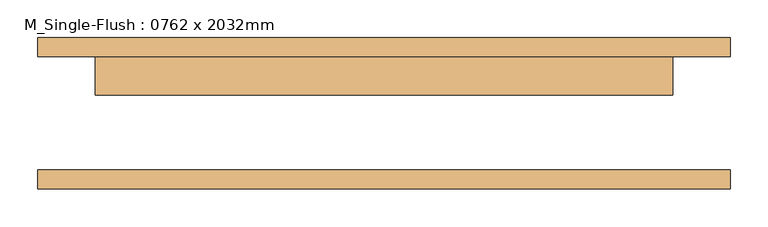
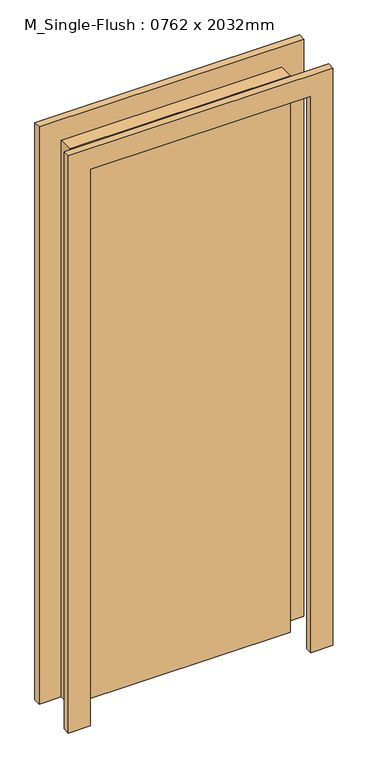
"""IFC4 building model written with IfcOpenShell, lengths in millimetres: door geometry, M_Single-Flush : 0762 x 2032mm."""

from ifc_helpers import new_model, si_unit, frame, origin, origin_with_axes, place, context, project, spatial, polyline, outline, extrude, source, transform, mapped, element, save


def m_single_flush_0762_x_2032mm_3f592dcc(model_context):
    return source(origin(), model_context, "Body", "SweptSolid", [
        extrude(outline(polyline([(2108.0, -457.0), (0.0, -457.0), (0.0, -381.0), (2032.0, -381.0), (2032.0, 381.0), (0.0, 381.0), (0.0, 457.0), (2108.0, 457.0), (2108.0, -457.0)])), frame((0.0, 75.0, 0.0), z_axis=(0.0, 1.0, 0.0), x_axis=(0.0, 0.0, 1.0)), (0.0, 0.0, 1.0), 25.0),
        extrude(outline(polyline([(2108.0, 457.0), (2108.0, -457.0), (0.0, -457.0), (0.0, -381.0), (2032.0, -381.0), (2032.0, 381.0), (0.0, 381.0), (0.0, 457.0), (2108.0, 457.0)])), frame((0.0, -100.0, 0.0), z_axis=(0.0, 1.0, 0.0), x_axis=(0.0, 0.0, 1.0)), (0.0, 0.0, 1.0), 25.0),
        extrude(outline(polyline([(381.0, 24.0), (-381.0, 24.0), (-381.0, 75.0), (381.0, 75.0), (381.0, 24.0)])), origin_with_axes(), (0.0, 0.0, 1.0), 2032.0),
    ])


if __name__ == "__main__":
    model = new_model("IFC4")
    model_context = context("Model", 3, world=origin())
    ifc_project = project(units=[si_unit("LENGTHUNIT", "METRE", prefix="MILLI")], contexts=[model_context])
    site = spatial("IfcSite", under=ifc_project)
    building = spatial("IfcBuilding", under=site)
    placement = place(None, origin())
    m_single_flush_0762_x_2032mm_shape = m_single_flush_0762_x_2032mm_3f592dcc(model_context)
    element("IfcDoor", 1, ObjectType="M_Single-Flush : 0762 x 2032mm", at=placement, inside=building, context=model_context, shape_type="MappedRepresentation", body=[
        mapped(m_single_flush_0762_x_2032mm_shape, transform((0.0, 0.0, 0.0), x_axis=(1.0, 0.0, 0.0), y_axis=(0.0, 1.0, 0.0), z_axis=(0.0, 0.0, 1.0))),
    ])
    save(model, "model.ifc")

# Revit data of these elements
# Type "M_Single-Flush : 0762 x 2032mm"
#   Type Mark = "19"
#   Thickness = 51 mm
#   Height = 2032 mm
#   Trim Projection Ext = 25 mm
#   Trim Projection Int = 25 mm
#   Trim Width = 76 mm
#   Width = 762 mm
#   Door Material = Door - Panel
#   Frame Material = Door - Frame
#   Function = (empty or 0)
#   Wall Closure = (empty or 0)
# Element 1 (IfcDoor, "M_Single-Flush : 0762 x 2032mm")
#   Materials on its faces: "Door - Frame", "Door - Panel"
# Materials
#   "Door - Panel": class "Wood", colour RGB 114 82 51, transparency 0
#   "Door - Frame": colour RGB 153 76 43, transparency 0
